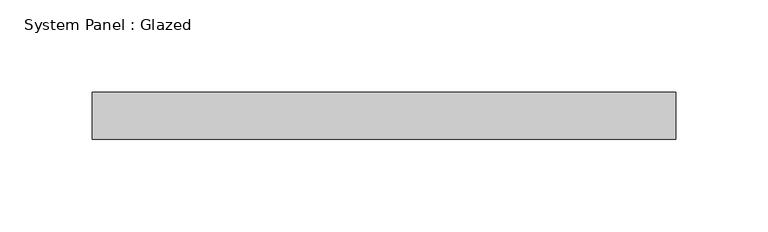
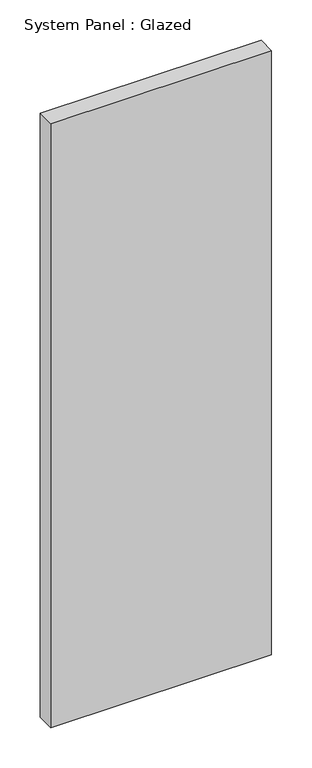
"""IFC4 building model written with IfcOpenShell, lengths in millimetres: plate geometry, System Panel : Glazed."""

from ifc_helpers import new_model, si_unit, origin, origin_with_axes, place, context, project, spatial, polyline, outline, extrude, source, transform, mapped, element, save


def system_panel_glazed_76d2efde(model_context):
    return source(origin(), model_context, "Body", "SweptSolid", [
        extrude(outline(polyline([(157.9957172, 19.05), (-157.9957172, 19.05), (-157.9957172, 44.45), (157.9957172, 44.45), (157.9957172, 19.05)])), origin_with_axes(), (0.0, 0.0, 1.0), 914.4),
    ])


if __name__ == "__main__":
    model = new_model("IFC4")
    model_context = context("Model", 3, world=origin())
    ifc_project = project(units=[si_unit("LENGTHUNIT", "METRE", prefix="MILLI")], contexts=[model_context])
    site = spatial("IfcSite", under=ifc_project)
    building = spatial("IfcBuilding", under=site)
    placement = place(None, origin())
    system_panel_glazed_shape = system_panel_glazed_76d2efde(model_context)
    element("IfcPlate", 1, ObjectType="System Panel : Glazed", at=placement, inside=building, context=model_context, shape_type="MappedRepresentation", body=[
        mapped(system_panel_glazed_shape, transform((0.0, 0.0, 0.0), x_axis=(1.0, 0.0, 0.0), y_axis=(0.0, 1.0, 0.0), z_axis=(0.0, 0.0, 1.0))),
    ])
    save(model, "model.ifc")

# Revit data of these elements
# Type "System Panel : Glazed"
#   Construction Type Id = "GSP4R"
#   Analytic Construction = "1/8 in Pilkington single glazing"
#   Visual Light Transmittance = 0.9
#   Solar Heat Gain Coefficient = 0.86
#   Heat Transfer Coefficient (U) = 1.18115 BTU/(h·ft²·°F)
# Element 1 (IfcPlate, "System Panel : Glazed")
#   Materials on its faces: "Glass"
# Materials
#   "Glass": class "Glass", colour RGB 0 128 192, transparency 0.75, Description = "Soda Lime Glass", Cost = 0
